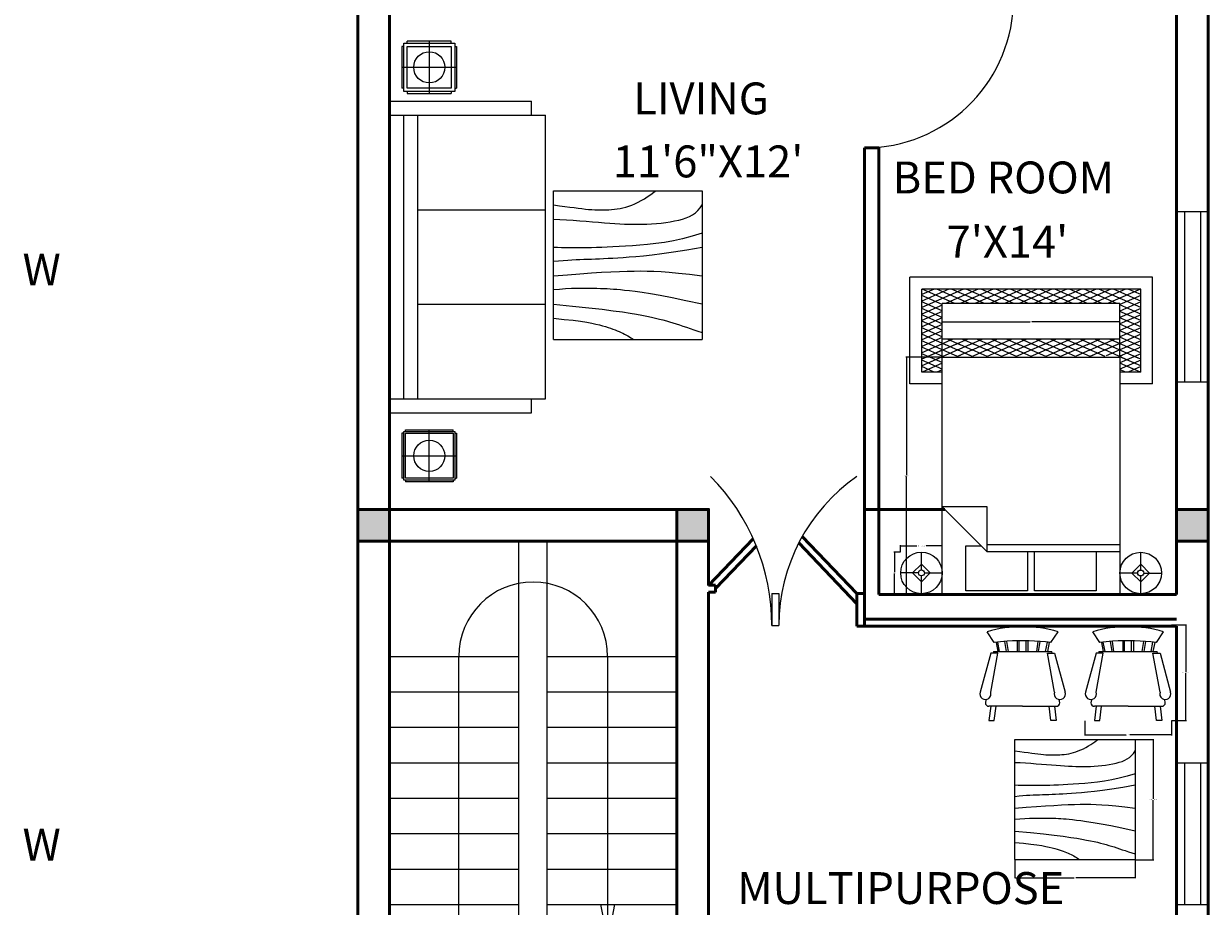
# Model space of a CAD drawing. Units: inches. Extents: x 28637 to 29820, y 17246 to 17928.
# Tile 4 of 6: x 28998 to 29332, y 17397 to 17646. Entities that reach past the tile are written whole.
import ezdxf

# ---------------------------------------------------------------- set-up
doc = ezdxf.new("R2010")
doc.units = ezdxf.units.IN
for name, color, linetype, lineweight in [('A-ANNO-DIMS', 2, 'Continuous', 18), ('A-ANNO-TEXT', 7, 'Continuous', 25), ('A-AREA-IDEN', 30, 'Continuous', 25), ('A-COLS', 1, 'Continuous', 50), ('A-DOOR', 4, 'Continuous', 25), ('A-FLOR-STRS', 3, 'Continuous', 25), ('A-FURN', 8, 'Continuous', 18), ('A-GLAZ', 4, 'Continuous', 25), ('A-WALL', 7, 'Continuous', 50)]:
    doc.layers.add(name, color=color, linetype=linetype, lineweight=lineweight)
doc.styles.get("Standard").update_dxf_attribs({"font": 'arial.ttf'})
doc.dimstyles.get("Standard").update_dxf_attribs({"dimtxt": 0.18, "dimasz": 0.18, "dimexe": 0.18, "dimexo": 0.0625, "dimgap": 0.09, "dimtad": 0, "dimtih": 1, "dimtoh": 1, "dimdec": 4, "dimzin": 0, "dimdsep": 46, "dimtxsty": 'Standard', "dimcen": 0.09, "dimadec": 0, "dimazin": 0, "dimtfac": 1, "dimtdec": 4, "dimtofl": 0, "dimtmove": 0, "dimatfit": 3, "dimfxl": 1, "dimtolj": 1, "dimtzin": 0, "dimarcsym": 0})

# ---------------------------------------------------------------- blocks, each defined once
blk = doc.blocks.new('Bed - Queen')
for p, q in [((0, -80.00003), (0, 0)), ((0, 0), (59.99999, 0)), ((59.99999, 0), (59.99999, -80.00003)), ((7.99999, -1.2), (28.79998, -1.2)), ((7.99999, -14.4), (7.99999, -1.2)), ((28.79998, -1.2), (28.79998, -14.4)), ((31.19999, -1.2), (51.99999, -1.2)), ((31.19999, -14.4), (31.19999, -1.2)), ((51.99999, -1.2), (51.99999, -16.4)), ((0, -14.4), (44.8, -14.4)), ((59.99999, -29.6), (44.8, -14.4)), ((44.8, -14.4), (44.8, -29.6)), ((44.8, -16.8), (0, -16.8)), ((51.99999, -16.4), (46.79936, -16.4)), ((44.8, -29.6), (59.99999, -29.6)), ((59.99999, -80.00003), (0, -80.00003))]:
    blk.add_line(p, q)
blk = doc.blocks.new('Lamp - Table')
for p, q in [((0, 7), (0, 1)), ((-1, 0), (-7, 0)), ((0, 3), (-3, 0)), ((-3, 0), (0, -3)), ((3, 0), (0, 3)), ((0, -3), (3, 0)), ((1, 0), (7, 0)), ((0, -1), (0, -7))]:
    blk.add_line(p, q)
for radius in [7, 1]:
    blk.add_circle((0, 0), radius)
blk = doc.blocks.new('Chair - Rocking')
for p, q in [((-8, -4.5), (-10, -1.5)), ((8, -4.5), (10, -1.5)), ((-7.5, -4.5), (-7, -7)), ((-6.5, -7), (-7.02225, -4.43)), ((-4.5, -7), (-4.96674, -4.19951)), ((-4, -7), (-4.40532, -4.16272)), ((-1.5, -4.05012), (-1.5, -7)), ((-1, -7), (-1, -4.05012)), ((1, -7), (1, -4.04655)), ((1.5, -4.05012), (1.5, -7)), ((4, -7), (4.40187, -4.18694)), ((4.5, -7), (4.96761, -4.19437)), ((6.5, -7), (7, -4.4057)), ((7.5, -4.5), (7, -7)), ((-9, -7.5), (-12, -18.49999)), ((-7, -7.5), (-9, -7.5)), ((-9, -18.49999), (-7, -7.5)), ((-8.23428, -6.99939), (-8.3093, -7.47958)), ((-8.23041, -7), (8.23915, -7)), ((7, -7.5), (9, -7.5)), ((9, -18.49999), (7, -7.5)), ((8.31071, -7.48854), (8.23449, -7.00073)), ((9, -7.5), (12, -18.49999)), ((-10.36644, -20.64523), (-10.5, -21.49999)), ((-9, -22.49999), (-9.5, -26.49999)), ((0, -22.49999), (-9.5, -22.49999)), ((-8, -26.49999), (-7.5, -22.49999)), ((0, -22.49999), (9.5, -22.49999)), ((8, -26.49999), (7.5, -22.49999)), ((9, -22.49999), (9.5, -26.49999)), ((10.5, -21.49999), (10.3575, -20.58798)), ((-9.5, -26.49999), (-8, -26.49999)), ((9.5, -26.49999), (8, -26.49999))]:
    blk.add_line(p, q)
for centre, radius, start, end in [((0, -34.08333), 34.08333, 72.93847, 107.0615), ((0, -68.25004), 64.25, 93.92211, 97.15267), ((0, -68.25004), 64.25, 82.84733, 93.92211), ((-10.5, -18.99999), 1.58114, 161.5651, 18.43495), ((10.5, -18.99999), 1.58114, 161.5651, 18.43495), ((-9.5, -21.49999), 1, 180, 270), ((9.5, -21.49999), 1, 270, 0)]:
    blk.add_arc(centre, radius, start, end)
blk = doc.blocks.new('Table - Square Woodgrain 42 x 42 in.')
blk.add_line((0, -42), (42, -42))
for points in [[(0, -4), (1.704, -4.2172), (3.2358, -4.4188), (4.615, -4.604), (5.8615, -4.7721), (6.9951, -4.9224), (8.0357, -5.0541), (9.0031, -5.1667), (9.9171, -5.2594), (10.7951, -5.3316), (11.6445, -5.3836), (12.4702, -5.4157), (13.277, -5.4283), (14.0698, -5.4217), (14.8535, -5.3964), (15.6331, -5.3526), (16.4133, -5.2908), (17.1986, -5.2103), (17.9913, -5.1062), (18.793, -4.9727), (19.6056, -4.8038), (20.4307, -4.5937), (21.2701, -4.3365), (22.1256, -4.0262), (22.9989, -3.6571), (23.888, -3.2272), (24.7756, -2.7516), (25.6408, -2.2491), (26.4624, -1.7387), (27.2195, -1.2395), (27.891, -0.7703), (28.456, -0.3501), (28.8934, 0.002)], [(0, -42), (0, 0), (42, 0), (42, -42)], [(0, -8), (1.8203, -8.1001), (3.6741, -8.2149), (5.5411, -8.3408), (7.4011, -8.4741), (9.2339, -8.6112), (11.0193, -8.7484), (12.7371, -8.8821), (14.3671, -9.0086), (15.8954, -9.1246), (17.3337, -9.2278), (18.6997, -9.3159), (20.0116, -9.387), (21.2871, -9.4389), (22.5442, -9.4696), (23.8008, -9.477), (25.0749, -9.459), (26.3791, -9.4137), (27.7049, -9.3403), (29.0383, -9.2382), (30.3655, -9.1068), (31.6728, -8.9455), (32.9461, -8.7535), (34.1717, -8.5304), (35.3358, -8.2756), (36.4268, -7.9863), (37.443, -7.6521), (38.3849, -7.2603), (39.253, -6.7986), (40.048, -6.2542), (40.7705, -5.6147), (41.421, -4.8674), (42, -4)], [(42, -12), (39.1784, -12.8621), (36.4519, -13.5654), (33.8246, -14.1294), (31.3004, -14.5731), (28.8832, -14.9161), (26.577, -15.1775), (24.3858, -15.3768), (22.3136, -15.5332), (20.3622, -15.6632), (18.5254, -15.7718), (16.7947, -15.8612), (15.1618, -15.9338), (13.6183, -15.9916), (12.1558, -16.0369), (10.7659, -16.0718), (9.4403, -16.0987), (8.1703, -16.1191), (6.9461, -16.1325), (5.7577, -16.1377), (4.595, -16.1335), (3.4479, -16.1188), (2.3064, -16.0924), (1.1604, -16.0532), (0, -16)], [(42, -16), (37.6529, -16.7365), (33.8802, -17.329), (30.6179, -17.7961), (27.8015, -18.1561), (25.3668, -18.4275), (23.2497, -18.6288), (21.3859, -18.7785), (19.7111, -18.8949), (18.1693, -18.9939), (16.7375, -19.0795), (15.401, -19.1534), (14.1449, -19.217), (12.9544, -19.2717), (11.8148, -19.3191), (10.7113, -19.3606), (9.6291, -19.3976), (8.5534, -19.4323), (7.47, -19.4689), (6.3643, -19.5122), (5.222, -19.5672), (4.0288, -19.6386), (2.7703, -19.7313), (1.4321, -19.8501), (0, -20)], [(0, -24), (3.9243, -23.6805), (7.4766, -23.4138), (10.6891, -23.1954), (13.5943, -23.0205), (16.2247, -22.8847), (18.6125, -22.7832), (20.7903, -22.7116), (22.7903, -22.6651), (24.6563, -22.642), (26.4764, -22.6507), (28.35, -22.7024), (30.3766, -22.8084), (32.6555, -22.98), (35.2861, -23.2283), (38.3678, -23.5645), (42, -24)], [(42, -32), (37.392, -31.017), (33.4585, -30.2231), (30.1291, -29.5949), (27.3334, -29.109), (25.0009, -28.742), (23.0612, -28.4707), (21.4439, -28.2716), (20.0786, -28.1215), (18.8998, -28.0002), (17.8609, -27.9014), (16.9206, -27.8219), (16.0371, -27.7588), (15.1691, -27.709), (14.2748, -27.6693), (13.3128, -27.6368), (12.2415, -27.6083), (11.0295, -27.5824), (9.6867, -27.5643), (8.233, -27.5608), (6.6884, -27.5787), (5.0728, -27.6248), (3.4062, -27.7058), (1.7086, -27.8286), (0, -28)], [(0, -32), (5.4026, -32.5358), (9.9494, -33.019), (13.7424, -33.4553), (16.8834, -33.8505), (19.4743, -34.2106), (21.6171, -34.5413), (23.4136, -34.8486), (24.9657, -35.1382), (26.3614, -35.4156), (27.6332, -35.6841), (28.7995, -35.9467), (29.8788, -36.2064), (30.8897, -36.4661), (31.8507, -36.7288), (32.7802, -36.9973), (33.6968, -37.2747), (34.6175, -37.5635), (35.5531, -37.8651), (36.5128, -38.1805), (37.506, -38.5108), (38.5421, -38.8568), (39.6302, -39.2197), (40.7797, -39.6004), (42, -40)], [(0, -36), (3.0098, -36.2857), (5.5354, -36.5643), (7.6368, -36.8359), (9.374, -37.1009), (10.807, -37.3597), (11.9957, -37.6126), (13.0002, -37.8599), (13.8804, -38.102), (14.6874, -38.3393), (15.4365, -38.5729), (16.1338, -38.8041), (16.7858, -39.0341), (17.3987, -39.264), (17.9787, -39.4952), (18.5322, -39.7288), (19.0655, -39.9662), (19.5832, -40.2081), (20.0842, -40.4544), (20.5657, -40.7046), (21.0249, -40.9581), (21.459, -41.2144), (21.8653, -41.4731), (22.2409, -41.7335), (22.5831, -41.9951)]]:
    blk.add_lwpolyline(points)
blk = doc.blocks.new('DOOR-42')
blk.add_line((28900.64, 17650.75), (28942.64, 17650.75))
blk.add_arc((28900.64, 17652.8), 42.05, 270, 357.2056)
blk = doc.blocks.new('DOOR-DOUBLE')
for p, q in [((17.27, 9), (17.27, 0)), ((17.27, 9), (19.27, 9)), ((19.27, 9), (19.27, 0)), ((19.27, 9), (19.27, 0)), ((17.27, 0), (19.27, 0))]:
    blk.add_line(p, q)
for centre, radius, start, end in [((-42.45, 0), 59.72, 0, 44.6951), ((70.36, 0), 51.09, 124.708, 180)]:
    blk.add_arc(centre, radius, start, end)
blk = doc.blocks.new('STAIR')
for p, q in [((28799.14, 17387.25), (28799.14, 17499.75)), ((28807.14, 17387.25), (28807.14, 17499.75)), ((28762.64, 17467.25), (28799.14, 17467.25)), ((28782.14, 17387.25), (28782.14, 17467.25)), ((28824.14, 17467.25), (28824.14, 17387.25)), ((28762.64, 17457.25), (28799.14, 17457.25)), ((28762.64, 17447.25), (28799.14, 17447.25)), ((28762.64, 17437.25), (28799.14, 17437.25)), ((28762.64, 17427.25), (28799.14, 17427.25)), ((28762.64, 17417.25), (28799.14, 17417.25)), ((28762.64, 17407.25), (28799.14, 17407.25)), ((28762.64, 17397.25), (28799.14, 17397.25)), ((28822.14, 17397.25), (28824.14, 17387.25)), ((28826.14, 17397.25), (28824.14, 17387.25)), ((28762.64, 17387.25), (28799.14, 17387.25))]:
    blk.add_line(p, q)
blk.add_arc((28803.14, 17467.25), 21, 0, 180)
blk = doc.blocks.new('SOFA-SET')
for p, q in [((28766.64, 17639.32), (28766.14, 17639.32)), ((28766.14, 17639.32), (28766.14, 17627.63)), ((28780.04, 17640.82), (28767.64, 17640.82)), ((28767.64, 17640.32), (28767.64, 17640.82)), ((28773.84, 17640.82), (28773.84, 17626.13)), ((28780.04, 17640.32), (28780.04, 17640.82)), ((28781.04, 17639.32), (28781.54, 17639.32)), ((28781.54, 17639.32), (28781.54, 17627.63)), ((28766.14, 17633.48), (28781.54, 17633.48)), ((28766.64, 17627.63), (28766.14, 17627.63)), ((28767.64, 17626.63), (28767.64, 17626.13)), ((28767.64, 17626.13), (28780.04, 17626.13)), ((28780.04, 17626.63), (28780.04, 17626.13)), ((28781.04, 17627.63), (28781.54, 17627.63)), ((28762.64, 17623.94), (28802.64, 17623.94)), ((28762.64, 17535.94), (28762.64, 17623.94)), ((28762.64, 17535.94), (28762.64, 17623.94)), ((28802.64, 17619.94), (28802.64, 17623.94)), ((28762.64, 17619.94), (28806.64, 17619.94)), ((28766.64, 17539.94), (28766.64, 17619.94)), ((28770.64, 17539.94), (28770.64, 17619.94)), ((28806.64, 17539.94), (28806.64, 17619.94)), ((28770.64, 17593.24), (28806.64, 17593.24)), ((28770.64, 17566.64), (28806.64, 17566.64)), ((28762.64, 17539.94), (28806.64, 17539.94)), ((28802.64, 17535.94), (28802.64, 17539.94)), ((28762.64, 17535.94), (28802.64, 17535.94)), ((28766.64, 17530.2), (28766.14, 17530.2)), ((28766.14, 17530.2), (28766.14, 17517.52)), ((28767.14, 17530.7), (28767.14, 17531.2)), ((28767.14, 17531.2), (28780.54, 17531.2)), ((28773.84, 17516.52), (28773.84, 17531.2)), ((28780.54, 17530.7), (28780.54, 17531.2)), ((28781.04, 17530.2), (28781.54, 17530.2)), ((28781.54, 17530.2), (28781.54, 17517.52)), ((28766.14, 17523.86), (28781.54, 17523.86)), ((28766.64, 17517.52), (28766.14, 17517.52)), ((28767.14, 17517.02), (28767.14, 17516.52)), ((28780.54, 17516.52), (28767.14, 17516.52)), ((28780.54, 17517.02), (28780.54, 17516.52)), ((28781.04, 17517.52), (28781.54, 17517.52))]:
    blk.add_line(p, q)
for points in [[(28766.64, 17640.32), (28781.04, 17640.32), (28781.04, 17626.63), (28766.64, 17626.63)], [(28767.64, 17639.32), (28780.04, 17639.32), (28780.04, 17627.63), (28767.64, 17627.63)], [(28766.64, 17530.7), (28781.04, 17530.7), (28781.04, 17517.02), (28766.64, 17517.02)], [(28767.14, 17530.2), (28780.54, 17530.2), (28780.54, 17517.52), (28767.14, 17517.52)]]:
    blk.add_lwpolyline(points, close=True)
for centre in [(28773.84, 17633.48), (28773.84, 17523.86)]:
    blk.add_circle(centre, 4.4)
blk = doc.blocks.new('*D22')
at = {"layer": 'A-ANNO-DIMS', "color": 0, "lineweight": -2, "transparency": 16777216}
for p, q in [((29256.71, 17551.65), (29246.56, 17551.65)), ((29246.74, 17551.47), (29246.74, 17518.39)), ((29246.74, 17484.93), (29246.74, 17518.01)), ((29256.71, 17484.75), (29246.56, 17484.75))]:
    blk.add_line(p, q, dxfattribs=at)
at = {"layer": 'A-ANNO-DIMS', "color": 0, "transparency": 16777216}
for points in [[(29246.71, 17551.47), (29246.77, 17551.47), (29246.74, 17551.65)], [(29246.71, 17484.93), (29246.77, 17484.93), (29246.74, 17484.75)]]:
    blk.add_solid(points, dxfattribs=at)
at = {"layer": 'Defpoints', "color": 0, "transparency": 16777216}
for p in [(29256.77, 17551.65), (29246.74, 17484.75), (29256.77, 17484.75)]:
    blk.add_point(p, dxfattribs=at)
at = {"layer": 'A-ANNO-DIMS', "color": 0, "transparency": 16777216, "insert": (29246.74, 17518.2), "char_height": 0.18, "attachment_point": 5}
blk.add_mtext('\\A1;QUEEN BED 67', dxfattribs=at)
blk = doc.blocks.new('*D23')
at = {"layer": 'A-ANNO-DIMS', "color": 0, "lineweight": -2, "transparency": 16777216}
for p, q in [((29256.77, 17551.71), (29256.77, 17561.86)), ((29256.95, 17561.68), (29281.64, 17561.68)), ((29306.76, 17561.68), (29282.08, 17561.68)), ((29306.94, 17551.71), (29306.94, 17561.86))]:
    blk.add_line(p, q, dxfattribs=at)
at = {"layer": 'A-ANNO-DIMS', "color": 0, "transparency": 16777216}
for points in [[(29256.95, 17561.71), (29256.95, 17561.65), (29256.77, 17561.68)], [(29306.76, 17561.71), (29306.76, 17561.65), (29306.94, 17561.68)]]:
    blk.add_solid(points, dxfattribs=at)
at = {"layer": 'Defpoints', "color": 0, "transparency": 16777216}
for p in [(29256.77, 17561.68), (29256.77, 17551.65), (29306.94, 17551.65)]:
    blk.add_point(p, dxfattribs=at)
at = {"layer": 'A-ANNO-DIMS', "color": 0, "transparency": 16777216, "insert": (29281.86, 17561.68), "char_height": 0.18, "attachment_point": 5}
blk.add_mtext('\\A1;50', dxfattribs=at)
blk = doc.blocks.new('*D28')
at = {"layer": 'A-ANNO-DIMS', "color": 0, "lineweight": -2, "transparency": 16777216}
for p, q in [((29245.06, 17496.72), (29245.06, 17498.6)), ((29245.24, 17498.42), (29249.58, 17498.42)), ((29256.59, 17498.42), (29252.26, 17498.42)), ((29256.77, 17496.72), (29256.77, 17498.6))]:
    blk.add_line(p, q, dxfattribs=at)
at = {"layer": 'A-ANNO-DIMS', "color": 0, "transparency": 16777216}
for points in [[(29245.24, 17498.45), (29245.24, 17498.39), (29245.06, 17498.42)], [(29256.59, 17498.45), (29256.59, 17498.39), (29256.77, 17498.42)]]:
    blk.add_solid(points, dxfattribs=at)
at = {"layer": 'Defpoints', "color": 0, "transparency": 16777216}
for p in [(29245.06, 17498.42), (29245.06, 17496.66), (29256.77, 17496.66)]:
    blk.add_point(p, dxfattribs=at)
at = {"layer": 'A-ANNO-DIMS', "color": 0, "transparency": 16777216, "insert": (29250.92, 17498.42), "char_height": 0.18, "attachment_point": 5}
blk.add_mtext('\\A1;TABLE LAMP 12 TYP.', dxfattribs=at)
blk = doc.blocks.new('*D29')
at = {"layer": 'A-ANNO-DIMS', "color": 0, "lineweight": -2, "transparency": 16777216}
for p, q in [((29245, 17496.66), (29243.13, 17496.66)), ((29243.31, 17496.48), (29243.31, 17490.99)), ((29243.31, 17485.13), (29243.31, 17490.63)), ((29245, 17484.95), (29243.13, 17484.95))]:
    blk.add_line(p, q, dxfattribs=at)
at = {"layer": 'A-ANNO-DIMS', "color": 0, "transparency": 16777216}
for points in [[(29243.28, 17496.48), (29243.34, 17496.48), (29243.31, 17496.66)], [(29243.28, 17485.13), (29243.34, 17485.13), (29243.31, 17484.95)]]:
    blk.add_solid(points, dxfattribs=at)
at = {"layer": 'Defpoints', "color": 0, "transparency": 16777216}
for p in [(29245.06, 17496.66), (29243.31, 17484.95), (29245.06, 17484.95)]:
    blk.add_point(p, dxfattribs=at)
at = {"layer": 'A-ANNO-DIMS', "color": 0, "transparency": 16777216, "insert": (29243.31, 17490.81), "char_height": 0.18, "attachment_point": 5}
blk.add_mtext('\\A1;12 TYP.', dxfattribs=at)
blk = doc.blocks.new('*D50')
at = {"layer": 'A-ANNO-DIMS', "color": 0, "lineweight": -2, "transparency": 16777216}
for p, q in [((29311.3, 17443.82), (29316.5, 17443.82)), ((29316.32, 17443.64), (29316.32, 17427.05)), ((29316.32, 17410.08), (29316.32, 17426.68)), ((29311.3, 17409.9), (29316.5, 17409.9))]:
    blk.add_line(p, q, dxfattribs=at)
at = {"layer": 'A-ANNO-DIMS', "color": 0, "transparency": 16777216}
for points in [[(29316.29, 17443.64), (29316.35, 17443.64), (29316.32, 17443.82)], [(29316.29, 17410.08), (29316.35, 17410.08), (29316.32, 17409.9)]]:
    blk.add_solid(points, dxfattribs=at)
at = {"layer": 'Defpoints', "color": 0, "transparency": 16777216}
for p in [(29311.23, 17443.82), (29316.32, 17443.82), (29311.23, 17409.9)]:
    blk.add_point(p, dxfattribs=at)
at = {"layer": 'A-ANNO-DIMS', "color": 0, "transparency": 16777216, "insert": (29316.32, 17426.86), "char_height": 0.18, "attachment_point": 5}
blk.add_mtext('\\A1;CENTER TABLE 34', dxfattribs=at)
blk = doc.blocks.new('*D51')
at = {"layer": 'A-ANNO-DIMS', "color": 0, "lineweight": -2, "transparency": 16777216}
for p, q in [((29277.32, 17409.84), (29277.32, 17404.64)), ((29311.23, 17409.84), (29311.23, 17404.64)), ((29277.5, 17404.82), (29294.06, 17404.82)), ((29311.05, 17404.82), (29294.49, 17404.82))]:
    blk.add_line(p, q, dxfattribs=at)
at = {"layer": 'A-ANNO-DIMS', "color": 0, "transparency": 16777216}
for points in [[(29277.5, 17404.85), (29277.5, 17404.79), (29277.32, 17404.82)], [(29311.05, 17404.85), (29311.05, 17404.79), (29311.23, 17404.82)]]:
    blk.add_solid(points, dxfattribs=at)
at = {"layer": 'Defpoints', "color": 0, "transparency": 16777216}
for p in [(29277.32, 17409.9), (29311.23, 17409.9), (29311.23, 17404.82)]:
    blk.add_point(p, dxfattribs=at)
at = {"layer": 'A-ANNO-DIMS', "color": 0, "transparency": 16777216, "insert": (29294.28, 17404.82), "char_height": 0.18, "attachment_point": 5}
blk.add_mtext('\\A1;34', dxfattribs=at)
blk = doc.blocks.new('*D52')
at = {"layer": 'A-ANNO-DIMS', "color": 0, "lineweight": -2, "transparency": 16777216}
for p, q in [((29321.52, 17476.17), (29325.69, 17476.17)), ((29325.51, 17475.99), (29325.51, 17462.85)), ((29325.51, 17449.35), (29325.51, 17462.49)), ((29321.52, 17449.17), (29325.69, 17449.17))]:
    blk.add_line(p, q, dxfattribs=at)
at = {"layer": 'A-ANNO-DIMS', "color": 0, "transparency": 16777216}
for points in [[(29325.48, 17475.99), (29325.54, 17475.99), (29325.51, 17476.17)], [(29325.48, 17449.35), (29325.54, 17449.35), (29325.51, 17449.17)]]:
    blk.add_solid(points, dxfattribs=at)
at = {"layer": 'Defpoints', "color": 0, "transparency": 16777216}
for p in [(29321.46, 17476.17), (29325.51, 17476.17), (29321.46, 17449.17)]:
    blk.add_point(p, dxfattribs=at)
at = {"layer": 'A-ANNO-DIMS', "color": 0, "transparency": 16777216, "insert": (29325.51, 17462.67), "char_height": 0.18, "attachment_point": 5}
blk.add_mtext('\\A1;ROCKING CHAIR 27 TYP.', dxfattribs=at)
blk = doc.blocks.new('*D53')
at = {"layer": 'A-ANNO-DIMS', "color": 0, "lineweight": -2, "transparency": 16777216}
for p, q in [((29297.02, 17449.11), (29297.02, 17444.94)), ((29321.46, 17449.11), (29321.46, 17444.94)), ((29297.2, 17445.12), (29308.71, 17445.12)), ((29321.28, 17445.12), (29309.77, 17445.12))]:
    blk.add_line(p, q, dxfattribs=at)
at = {"layer": 'A-ANNO-DIMS', "color": 0, "transparency": 16777216}
for points in [[(29297.2, 17445.15), (29297.2, 17445.09), (29297.02, 17445.12)], [(29321.28, 17445.15), (29321.28, 17445.09), (29321.46, 17445.12)]]:
    blk.add_solid(points, dxfattribs=at)
at = {"layer": 'Defpoints', "color": 0, "transparency": 16777216}
for p in [(29297.02, 17449.17), (29321.46, 17449.17), (29321.46, 17445.12)]:
    blk.add_point(p, dxfattribs=at)
at = {"layer": 'A-ANNO-DIMS', "color": 0, "transparency": 16777216, "insert": (29309.24, 17445.12), "char_height": 0.18, "attachment_point": 5}
blk.add_mtext('\\A1;24 TYP.', dxfattribs=at)

msp = doc.modelspace()

# ---------------------------------------------------------------- hatches: boundary and pattern name
at = {"layer": 'A-COLS'}
h = msp.add_hatch(color=256, dxfattribs=at)
h.dxf.hatch_style = 1
h.paths.add_polyline_path([(29091.87, 17508.75), (29091.87, 17499.75), (29100.87, 17499.75), (29100.87, 17508.75)])
h = msp.add_hatch(color=256, dxfattribs=at)
h.dxf.hatch_style = 1
h.paths.add_polyline_path([(29181.87, 17508.75), (29181.87, 17499.75), (29190.87, 17499.75), (29190.87, 17508.75)])
h = msp.add_hatch(color=256, dxfattribs=at)
h.dxf.hatch_style = 1
h.paths.add_polyline_path([(29322.87, 17508.75), (29322.87, 17499.75), (29331.87, 17499.75), (29331.87, 17508.75)])

# ---------------------------------------------------------------- linework, layer by layer
for points in [[(29091.87, 17508.75), (29100.87, 17508.75), (29100.87, 17499.75), (29091.87, 17499.75)], [(29181.87, 17508.75), (29190.87, 17508.75), (29190.87, 17499.75), (29181.87, 17499.75)], [(29322.87, 17508.75), (29331.87, 17508.75), (29331.87, 17499.75), (29322.87, 17499.75)]]:
    msp.add_lwpolyline(points, close=True, dxfattribs=at)
at = {"layer": 'A-FLOR-STRS'}
for p, q in [((29145.37, 17467.25), (29181.87, 17467.25)), ((29145.37, 17457.25), (29181.87, 17457.25)), ((29145.37, 17447.25), (29181.87, 17447.25)), ((29145.37, 17437.25), (29181.87, 17437.25)), ((29145.37, 17427.25), (29181.87, 17427.25)), ((29145.37, 17417.25), (29181.87, 17417.25)), ((29145.37, 17407.25), (29181.87, 17407.25)), ((29145.37, 17397.25), (29181.87, 17397.25))]:
    msp.add_line(p, q, dxfattribs=at)
at = {"layer": 'A-FURN'}
for p, q in [((29316.14, 17574.24), (29247.66, 17574.24)), ((29247.66, 17544.14), (29247.66, 17574.24)), ((29316.14, 17544.14), (29316.14, 17574.24)), ((29312.8, 17570.89), (29251.01, 17570.89)), ((29262.82, 17570.89), (29251.01, 17565.7)), ((29258.66, 17570.89), (29251.01, 17567.53)), ((29254.51, 17570.89), (29251.01, 17569.35)), ((29251.01, 17547.48), (29251.01, 17570.89)), ((29256.77, 17566.58), (29251.01, 17569.11)), ((29260.37, 17566.82), (29251.11, 17570.89)), ((29264.53, 17566.82), (29255.27, 17570.89)), ((29264.53, 17566.82), (29255.27, 17570.89)), ((29266.97, 17570.89), (29257.71, 17566.82)), ((29268.68, 17566.82), (29259.43, 17570.89)), ((29271.13, 17570.89), (29261.87, 17566.82)), ((29272.84, 17566.82), (29263.58, 17570.89)), ((29275.29, 17570.89), (29266.03, 17566.82)), ((29277, 17566.82), (29267.74, 17570.89)), ((29279.44, 17570.89), (29270.18, 17566.82)), ((29281.15, 17566.82), (29271.89, 17570.89)), ((29283.6, 17570.89), (29274.34, 17566.82)), ((29285.31, 17566.82), (29276.05, 17570.89)), ((29287.75, 17570.89), (29278.49, 17566.82)), ((29289.46, 17566.82), (29280.21, 17570.89)), ((29291.91, 17570.89), (29282.65, 17566.82)), ((29293.62, 17566.82), (29284.36, 17570.89)), ((29296.07, 17570.89), (29286.81, 17566.82)), ((29297.78, 17566.82), (29288.52, 17570.89)), ((29300.22, 17570.89), (29290.96, 17566.82)), ((29300.22, 17570.89), (29290.96, 17566.82)), ((29301.93, 17566.82), (29292.67, 17570.89)), ((29304.38, 17570.89), (29295.12, 17566.82)), ((29304.38, 17570.89), (29295.12, 17566.82)), ((29304.38, 17570.89), (29295.12, 17566.82)), ((29306.09, 17566.82), (29296.83, 17570.89)), ((29308.53, 17570.89), (29299.27, 17566.82)), ((29312.8, 17565.7), (29300.98, 17570.89)), ((29312.69, 17570.89), (29303.43, 17566.82)), ((29312.8, 17567.53), (29305.14, 17570.89)), ((29312.8, 17569.11), (29306.94, 17566.54)), ((29312.8, 17569.35), (29309.3, 17570.89)), ((29312.8, 17547.48), (29312.8, 17570.89)), ((29256.77, 17564.75), (29251.01, 17567.29)), ((29256.77, 17566.41), (29251.01, 17563.87)), ((29256.77, 17562.93), (29251.01, 17565.46)), ((29306.94, 17566.82), (29256.77, 17566.82)), ((29256.77, 17556.79), (29256.77, 17566.82)), ((29312.8, 17567.29), (29306.94, 17564.71)), ((29306.94, 17556.79), (29306.94, 17566.82)), ((29312.8, 17563.87), (29306.94, 17566.45)), ((29312.8, 17565.46), (29306.94, 17562.89)), ((29256.77, 17564.58), (29251.01, 17562.05)), ((29256.77, 17561.1), (29251.01, 17563.63)), ((29256.77, 17562.75), (29251.01, 17560.22)), ((29256.77, 17559.27), (29251.01, 17561.81)), ((29312.8, 17562.05), (29306.94, 17564.62)), ((29312.8, 17563.63), (29306.94, 17561.06)), ((29312.8, 17560.22), (29306.94, 17562.79)), ((29312.8, 17561.81), (29306.94, 17559.23)), ((29256.77, 17560.93), (29251.01, 17558.39)), ((29256.77, 17557.45), (29251.01, 17559.98)), ((29256.77, 17559.1), (29251.01, 17556.57)), ((29312.8, 17558.39), (29306.94, 17560.97)), ((29312.8, 17559.98), (29306.94, 17557.41)), ((29312.8, 17556.57), (29306.94, 17559.14)), ((29257.91, 17555.12), (29251.01, 17558.15)), ((29256.77, 17557.27), (29251.01, 17554.74)), ((29259.82, 17556.79), (29251.01, 17552.91)), ((29257.24, 17553.59), (29251.01, 17556.33)), ((29261.12, 17551.88), (29251.01, 17556.33)), ((29260.5, 17555.26), (29251.68, 17551.38)), ((29306.94, 17556.79), (29256.77, 17556.79)), ((29261.4, 17553.59), (29257.59, 17555.26)), ((29261.4, 17553.59), (29257.59, 17555.26)), ((29262.07, 17555.12), (29258.26, 17556.79)), ((29263.98, 17556.79), (29260.17, 17555.12)), ((29264.65, 17555.26), (29260.85, 17553.59)), ((29264.65, 17555.26), (29260.85, 17553.59)), ((29265.55, 17553.59), (29261.75, 17555.26)), ((29266.23, 17555.12), (29262.42, 17556.79)), ((29268.13, 17556.79), (29264.33, 17555.12)), ((29268.13, 17556.79), (29264.33, 17555.12)), ((29268.81, 17555.26), (29265, 17553.59)), ((29269.71, 17553.59), (29265.9, 17555.26)), ((29270.38, 17555.12), (29266.58, 17556.79)), ((29272.29, 17556.79), (29268.49, 17555.12)), ((29272.29, 17556.79), (29268.49, 17555.12)), ((29272.29, 17556.79), (29268.49, 17555.12)), ((29272.96, 17555.26), (29269.16, 17553.59)), ((29277.12, 17555.26), (29269.43, 17551.88)), ((29273.86, 17553.59), (29270.06, 17555.26)), ((29274.54, 17555.12), (29270.73, 17556.79)), ((29276.45, 17556.79), (29272.64, 17555.12)), ((29281.28, 17555.26), (29273.52, 17551.85)), ((29278.02, 17553.59), (29274.22, 17555.26)), ((29278.69, 17555.12), (29274.89, 17556.79)), ((29280.6, 17556.79), (29276.8, 17555.12)), ((29285.43, 17555.26), (29277.68, 17551.85)), ((29282.18, 17553.59), (29278.37, 17555.26)), ((29282.85, 17555.12), (29279.04, 17556.79)), ((29284.76, 17556.79), (29280.95, 17555.12)), ((29289.59, 17555.26), (29281.83, 17551.85)), ((29286.33, 17553.59), (29282.53, 17555.26)), ((29287, 17555.12), (29283.2, 17556.79)), ((29288.91, 17556.79), (29285.11, 17555.12)), ((29293.74, 17555.26), (29285.99, 17551.85)), ((29290.49, 17553.59), (29286.68, 17555.26)), ((29291.16, 17555.12), (29287.36, 17556.79)), ((29291.16, 17555.12), (29287.36, 17556.79)), ((29293.07, 17556.79), (29289.27, 17555.12)), ((29293.07, 17556.79), (29289.27, 17555.12)), ((29293.07, 17556.79), (29289.27, 17555.12)), ((29297.9, 17555.26), (29290.21, 17551.88)), ((29294.64, 17553.59), (29290.84, 17555.26)), ((29295.32, 17555.12), (29291.51, 17556.79)), ((29297.23, 17556.79), (29293.42, 17555.12)), ((29302.75, 17551.85), (29294.37, 17555.53)), ((29302.68, 17553.71), (29295.67, 17556.79)), ((29301.38, 17556.79), (29297.58, 17555.12)), ((29302.05, 17555.26), (29298.25, 17553.59)), ((29306.21, 17555.26), (29298.46, 17551.85)), ((29303.63, 17555.12), (29299.82, 17556.79)), ((29305.54, 17556.79), (29301.73, 17555.12)), ((29306.21, 17555.26), (29302.41, 17553.59)), ((29306.21, 17555.26), (29302.41, 17553.59)), ((29312.12, 17551.38), (29303.31, 17555.26)), ((29312.8, 17552.91), (29303.98, 17556.79)), ((29312.8, 17558.15), (29305.89, 17555.12)), ((29312.8, 17554.74), (29306.94, 17557.31)), ((29312.8, 17556.33), (29306.94, 17553.75)), ((29256.1, 17552.26), (29251.01, 17554.5)), ((29256.1, 17552.26), (29251.01, 17554.5)), ((29256.97, 17551.88), (29251.01, 17554.5)), ((29256.77, 17553.62), (29251.01, 17551.09)), ((29256.77, 17550.14), (29251.01, 17552.67)), ((29256.77, 17551.79), (29251.01, 17549.26)), ((29256.77, 17551.79), (29251.01, 17549.26)), ((29261.17, 17553.73), (29252.35, 17549.85)), ((29261.17, 17553.73), (29252.35, 17549.85)), ((29261.19, 17551.85), (29260.4, 17552.2)), ((29261.84, 17552.2), (29261.05, 17551.85)), ((29264.88, 17552.05), (29261.07, 17553.73)), ((29265.28, 17551.88), (29261.07, 17553.73)), ((29265.32, 17553.73), (29261.52, 17552.05)), ((29266, 17552.2), (29265.21, 17551.85)), ((29269.5, 17551.85), (29265.23, 17553.73)), ((29269.48, 17553.73), (29265.68, 17552.05)), ((29273.59, 17551.88), (29269.39, 17553.73)), ((29277.75, 17551.88), (29271.51, 17554.62)), ((29281.9, 17551.88), (29277.7, 17553.73)), ((29286.06, 17551.88), (29279.82, 17554.62)), ((29289.81, 17552.05), (29286.01, 17553.73)), ((29290.28, 17551.85), (29289.49, 17552.2)), ((29294.44, 17551.85), (29290.17, 17553.73)), ((29298.52, 17551.88), (29292.29, 17554.62)), ((29298.57, 17553.73), (29294.37, 17551.88)), ((29298.57, 17553.73), (29294.77, 17552.05)), ((29299.25, 17552.2), (29298.46, 17551.85)), ((29302.75, 17551.85), (29301.96, 17552.2)), ((29311.45, 17549.85), (29302.63, 17553.73)), ((29306.88, 17553.73), (29303.08, 17552.05)), ((29306.88, 17553.73), (29303.08, 17552.05)), ((29307.56, 17552.2), (29306.77, 17551.85)), ((29312.8, 17554.5), (29306.94, 17551.93)), ((29312.8, 17551.09), (29306.94, 17553.66)), ((29312.8, 17552.67), (29306.94, 17550.1)), ((29312.8, 17549.26), (29306.94, 17551.83)), ((29256.77, 17548.31), (29251.01, 17550.85)), ((29254.51, 17547.48), (29251.01, 17549.02)), ((29256.77, 17549.97), (29251.11, 17547.48)), ((29256.77, 17549.97), (29251.11, 17547.48)), ((29256.77, 17549.97), (29251.11, 17547.48)), ((29256.77, 17549.97), (29253.02, 17548.32)), ((29312.8, 17550.85), (29306.94, 17548.27)), ((29312.69, 17547.48), (29306.94, 17550.01)), ((29310.78, 17548.32), (29306.94, 17550.01)), ((29312.8, 17549.02), (29309.3, 17547.48)), ((29256.77, 17547.48), (29251.01, 17547.48)), ((29256.77, 17548.14), (29255.27, 17547.48)), ((29308.53, 17547.48), (29306.94, 17548.18)), ((29308.53, 17547.48), (29306.94, 17548.18)), ((29312.8, 17547.48), (29306.94, 17547.48)), ((29256.77, 17544.14), (29247.66, 17544.14)), ((29316.14, 17544.14), (29306.94, 17544.14))]:
    msp.add_line(p, q, dxfattribs=at)
at = {"layer": 'A-GLAZ'}
for p, q in [((29322.87, 17592.75), (29331.87, 17592.75)), ((29325.12, 17592.75), (29325.12, 17544.75)), ((29329.62, 17592.75), (29329.62, 17544.75)), ((29322.87, 17544.75), (29331.87, 17544.75)), ((29322.87, 17437.25), (29331.87, 17437.25)), ((29325.12, 17437.25), (29325.12, 17397.25)), ((29329.62, 17437.25), (29329.62, 17397.25)), ((29322.87, 17397.25), (29331.87, 17397.25))]:
    msp.add_line(p, q, dxfattribs=at)
at = {"layer": 'A-WALL'}
for p, q in [((29091.87, 17334.75), (29091.87, 17814.75)), ((29331.87, 17814.75), (29331.87, 17334.75)), ((29100.87, 17508.75), (29100.87, 17652.75)), ((29322.87, 17652.75), (29322.87, 17484.75)), ((29322.87, 17652.75), (29322.87, 17484.75)), ((29234.87, 17610.75), (29238.87, 17610.75)), ((29234.87, 17610.75), (29234.87, 17477.75)), ((29234.87, 17610.75), (29234.87, 17475.75)), ((29238.87, 17610.75), (29238.87, 17484.75)), ((29091.87, 17508.75), (29190.87, 17508.75)), ((29190.87, 17508.75), (29190.87, 17487.26)), ((29234.87, 17508.75), (29257.52, 17508.75)), ((29100.87, 17499.75), (29181.87, 17499.75)), ((29100.87, 17343.75), (29100.87, 17499.75)), ((29181.87, 17499.75), (29181.87, 17387.25)), ((29190.87, 17487.26), (29203.49, 17500.45)), ((29192.83, 17486.42), (29204.35, 17498.45)), ((29232.72, 17482.12), (29216.32, 17499.27)), ((29232.72, 17485.02), (29217.31, 17501.12)), ((29190.83, 17487.35), (29192.83, 17487.35)), ((29190.83, 17485.35), (29192.83, 17485.35)), ((29190.87, 17485.35), (29190.87, 17387.25)), ((29192.83, 17487.35), (29192.83, 17485.35)), ((29232.72, 17485.02), (29234.72, 17485.02)), ((29232.72, 17485.02), (29232.72, 17475.75)), ((29238.87, 17484.75), (29322.87, 17484.75)), ((29208.7, 17477.75), (29208.72, 17477.75)), ((29210.72, 17477.75), (29210.75, 17477.75)), ((29232.72, 17475.75), (29322.87, 17475.75)), ((29234.87, 17477.75), (29322.87, 17477.75)), ((29322.87, 17475.75), (29322.87, 17343.75)), ((29322.87, 17475.75), (29322.87, 17397.25))]:
    msp.add_line(p, q, dxfattribs=at)

# ---------------------------------------------------------------- block references
at = {"layer": 'A-DOOR'}
for name, p in [('DOOR-42', (334.22, 0)), ('DOOR-DOUBLE', (29191.45, 17476.02))]:
    msp.add_blockref(name, p, dxfattribs=at)
at = {"layer": 'A-FLOR-STRS'}
msp.add_blockref('STAIR', (338.22, 0), dxfattribs=at)
at = {"layer": 'A-FURN'}
for name, p in [('SOFA-SET', (338.22, 0)), ('Table - Square Woodgrain 42 x 42 in.', (29147.1, 17598.65)), ('Chair - Rocking', (29279.47, 17475.67)), ('Chair - Rocking', (29309.24, 17475.67))]:
    msp.add_blockref(name, p, dxfattribs=at)
at = {"layer": 'A-FURN', "xscale": 0.8362135169518563, "yscale": 0.8362135169518563, "zscale": 0.8362135169518563, "rotation": 180}
for name, p in [('Bed - Queen', (29306.94, 17484.75)), ('Lamp - Table', (29250.92, 17490.81)), ('Lamp - Table', (29312.8, 17490.79))]:
    msp.add_blockref(name, p, dxfattribs=at)
at = {"layer": 'A-FURN', "xscale": 0.8074778780150476, "yscale": 0.8074778780150476, "zscale": 0.8074778780150476}
msp.add_blockref('Table - Square Woodgrain 42 x 42 in.', (29277.32, 17443.82), dxfattribs=at)

# ---------------------------------------------------------------- texts
at = {"layer": 'A-ANNO-TEXT'}
for p in [(28986.3, 17571.93), (28986.3, 17409.66)]:
    msp.add_text('    W', height=9, dxfattribs=at).set_placement(p)
at = {"layer": 'A-AREA-IDEN'}
for s, p in [('LIVING', (29169.59, 17620.2)), (' 11\'6"X12\'', (29161.1, 17602.42)), ('BED ROOM', (29242.8, 17597.9)), ("   7'X14'", (29249.79, 17579.78)), ('MULTIPURPOSE', (29198.95, 17397.39))]:
    msp.add_text(s, height=9, dxfattribs=at).set_placement(p)

# ---------------------------------------------------------------- dimensions: what is measured, and where the dimension line sits
at = {"layer": 'A-ANNO-DIMS'}
dim = msp.add_linear_dim(base=(29256.77, 17561.68), p1=(29306.94, 17551.65), p2=(29256.77, 17551.65), angle=180, dimstyle='Standard', override={"dimdec": 0, "dimlfac": 1, "dimrnd": 0, "dimzin": 0, "dimdsep": 46, "dimlunit": 2}, dxfattribs=at)
dim.commit()
dim.dimension.update_dxf_attribs({"geometry": '*D23', "text_midpoint": (29281.86, 17561.68)})
for base, p1, p2, angle, text, picture, middle in [((29246.74, 17484.75), (29256.77, 17551.65), (29256.77, 17484.75), 270, 'QUEEN BED <>', '*D22', (29246.74, 17518.2)), ((29245.06, 17498.42), (29256.77, 17496.66), (29245.06, 17496.66), 180, 'TABLE LAMP <> TYP.', '*D28', (29250.92, 17498.42)), ((29243.31, 17484.95), (29245.06, 17496.66), (29245.06, 17484.95), 270, '<> TYP.', '*D29', (29243.31, 17490.81)), ((29325.51, 17476.17), (29321.46, 17449.17), (29321.46, 17476.17), 90, 'ROCKING CHAIR <> TYP.', '*D52', (29325.51, 17462.67)), ((29316.32, 17443.82), (29311.23, 17409.9), (29311.23, 17443.82), 90, 'CENTER TABLE <>', '*D50', (29316.32, 17426.86))]:
    dim = msp.add_linear_dim(base=base, p1=p1, p2=p2, angle=angle, text=text, dimstyle='Standard', override={"dimdec": 0, "dimlfac": 1, "dimrnd": 0, "dimzin": 0, "dimdsep": 46, "dimlunit": 2}, dxfattribs=at)
    dim.commit()
    dim.dimension.update_dxf_attribs({"geometry": picture, "text_midpoint": middle})
dim = msp.add_linear_dim(base=(29321.46, 17445.12), p1=(29297.02, 17449.17), p2=(29321.46, 17449.17), text='<> TYP.', dimstyle='Standard', override={"dimdec": 0, "dimlfac": 1, "dimrnd": 0, "dimzin": 0, "dimdsep": 46, "dimlunit": 2}, dxfattribs=at)
dim.commit()
dim.dimension.update_dxf_attribs({"geometry": '*D53', "text_midpoint": (29309.24, 17445.12)})
dim = msp.add_linear_dim(base=(29311.23, 17404.82), p1=(29277.32, 17409.9), p2=(29311.23, 17409.9), dimstyle='Standard', override={"dimdec": 0, "dimlfac": 1, "dimrnd": 0, "dimzin": 0, "dimdsep": 46, "dimlunit": 2}, dxfattribs=at)
dim.commit()
dim.dimension.update_dxf_attribs({"geometry": '*D51', "text_midpoint": (29294.28, 17404.82)})

doc.saveas('drawing.dxf')
